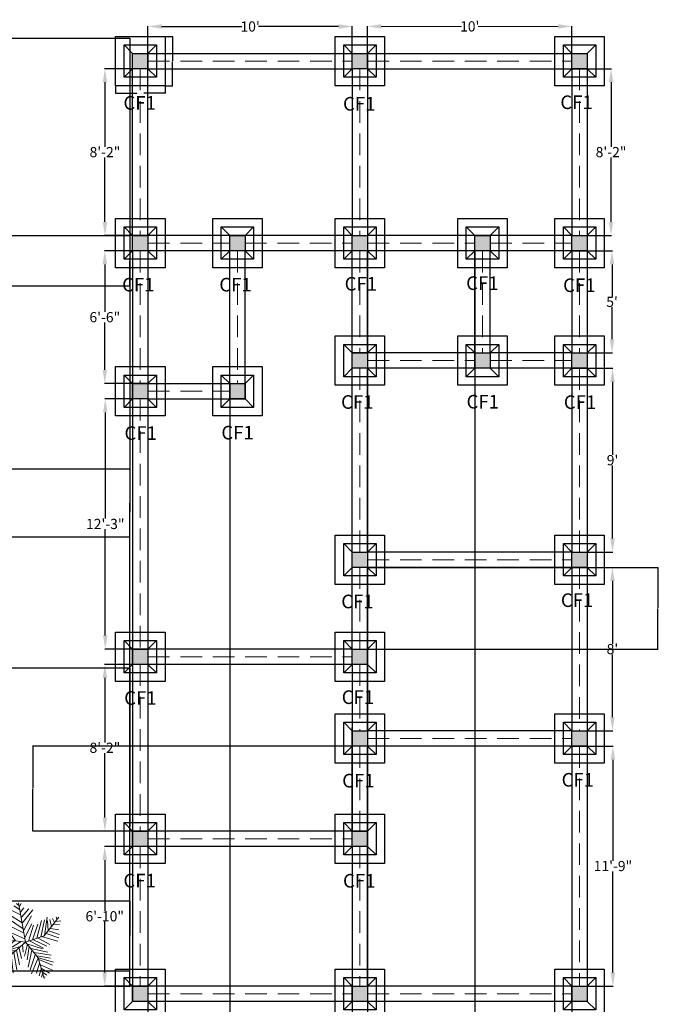
# Model space of a CAD drawing. Units: inches. Extents: x 37 to 824, y -700 to 234.
# Tile 77 of 77: x 449 to 824, y -377 to 202. Entities that reach past the tile are written whole.
import ezdxf

# ---------------------------------------------------------------- set-up
doc = ezdxf.new("R2010")
doc.units = ezdxf.units.IN
doc.header["$MEASUREMENT"] = 0
doc.linetypes.add('DASHED', pattern=[19.05, 12.7, -6.35])
for name, color, linetype, lineweight in [('A-ANNO-DIMS', 2, 'Continuous', 18), ('A-ANNO-TEXT', 7, 'Continuous', 18), ('A-SITE-PLNT', 3, 'Continuous', 13), ('S-BEAM', 4, 'Continuous', 25), ('S-BEAM-CNTR', 220, 'DASHED', 18), ('S-COLS', 2, 'Continuous', 35), ('S-FNDN', 220, 'Continuous', 25)]:
    doc.layers.add(name, color=color, linetype=linetype, lineweight=lineweight)
doc.styles.get("Standard").update_dxf_attribs({"font": 'arial.ttf'})
doc.dimstyles.get("Standard").update_dxf_attribs({"dimtxt": 0.18, "dimasz": 0.18, "dimexe": 0.18, "dimexo": 0.0625, "dimgap": 0.09, "dimtad": 0, "dimtih": 1, "dimtoh": 1, "dimdec": 1, "dimzin": 0, "dimdsep": 46, "dimlunit": 4, "dimtxsty": 'Standard', "dimcen": 0.09, "dimadec": 0, "dimazin": 0, "dimtfac": 1, "dimtdec": 1, "dimtofl": 0, "dimtmove": 0, "dimatfit": 3, "dimfxl": 1, "dimtolj": 1, "dimtzin": 0, "dimarcsym": 0})

# ---------------------------------------------------------------- blocks, each defined once
blk = doc.blocks.new('*D12')
at = {"layer": 'A-ANNO-DIMS', "color": 0, "lineweight": -2, "ltscale": 0.5, "transparency": 16777216}
for p, q in [((524.2, 173.16), (524.2, 198.08)), ((532.2, 197.9), (579.3, 197.9)), ((636.2, 197.9), (589.1, 197.9)), ((644.2, 173.16), (644.2, 198.08))]:
    blk.add_line(p, q, dxfattribs=at)
at = {"layer": 'A-ANNO-DIMS', "color": 0, "ltscale": 0.5, "transparency": 16777216}
for points in [[(532.2, 199.23), (532.2, 196.56), (524.2, 197.9)], [(636.2, 199.23), (636.2, 196.56), (644.2, 197.9)]]:
    blk.add_solid(points, dxfattribs=at)
at = {"layer": 'Defpoints', "color": 0, "ltscale": 0.5, "transparency": 16777216}
for p in [(644.2, 197.9), (524.2, 173.09), (644.2, 173.09)]:
    blk.add_point(p, dxfattribs=at)
at = {"layer": 'A-ANNO-DIMS', "color": 0, "ltscale": 0.5, "transparency": 16777216, "insert": (584.2, 197.9), "char_height": 6, "attachment_point": 5}
blk.add_mtext("\\A1;10'", dxfattribs=at)
blk = doc.blocks.new('*D13')
at = {"layer": 'A-ANNO-DIMS', "color": 0, "lineweight": -2, "ltscale": 0.5, "transparency": 16777216}
for p, q in [((653.2, 173.16), (653.2, 198.13)), ((773.2, 173.16), (773.2, 198.13))]:
    blk.add_line(p, q, dxfattribs=at)
at = {"layer": 'A-ANNO-DIMS', "color": 0, "ltscale": 0.5, "transparency": 16777216}
for p, q in [((661.2, 197.95), (708.3, 197.95)), ((765.2, 197.95), (718.1, 197.95))]:
    blk.add_line(p, q, dxfattribs=at)
for points in [[(661.2, 199.28), (661.2, 196.62), (653.2, 197.95)], [(765.2, 199.28), (765.2, 196.62), (773.2, 197.95)]]:
    blk.add_solid(points, dxfattribs=at)
at = {"layer": 'Defpoints', "color": 0, "ltscale": 0.5, "transparency": 16777216}
for p in [(773.2, 197.95), (653.2, 173.09), (773.2, 173.09)]:
    blk.add_point(p, dxfattribs=at)
at = {"layer": 'A-ANNO-DIMS', "color": 0, "ltscale": 0.5, "transparency": 16777216, "insert": (713.2, 197.95), "char_height": 6, "attachment_point": 5}
blk.add_mtext("\\A1;10'", dxfattribs=at)
blk = doc.blocks.new('*D14')
at = {"layer": 'A-ANNO-DIMS', "color": 0, "lineweight": -2, "ltscale": 0.5, "transparency": 16777216}
for p, q in [((773.26, 173.09), (796.39, 173.09)), ((796.21, 165.09), (796.21, 127.25)), ((796.21, 83.09), (796.21, 120.94)), ((773.26, 75.09), (796.39, 75.09))]:
    blk.add_line(p, q, dxfattribs=at)
at = {"layer": 'A-ANNO-DIMS', "color": 0, "ltscale": 0.5, "transparency": 16777216}
for points in [[(794.88, 165.09), (797.55, 165.09), (796.21, 173.09)], [(794.88, 83.09), (797.55, 83.09), (796.21, 75.09)]]:
    blk.add_solid(points, dxfattribs=at)
at = {"layer": 'Defpoints', "color": 0, "ltscale": 0.5, "transparency": 16777216}
for p in [(773.2, 173.09), (773.2, 75.09), (796.21, 75.09)]:
    blk.add_point(p, dxfattribs=at)
at = {"layer": 'A-ANNO-DIMS', "color": 0, "ltscale": 0.5, "transparency": 16777216, "insert": (796.21, 124.09), "char_height": 6, "attachment_point": 5}
blk.add_mtext('\\A1;8\'-2"', dxfattribs=at)
blk = doc.blocks.new('*D15')
at = {"layer": 'A-ANNO-DIMS', "color": 0, "lineweight": -2, "ltscale": 0.6, "transparency": 16777216}
for p, q in [((773.26, 66.09), (796.98, 66.09)), ((796.8, 58.09), (796.8, 39.23)), ((796.8, 14.09), (796.8, 32.95)), ((773.26, 6.09), (796.98, 6.09))]:
    blk.add_line(p, q, dxfattribs=at)
at = {"layer": 'A-ANNO-DIMS', "color": 0, "ltscale": 0.6, "transparency": 16777216}
for points in [[(795.47, 58.09), (798.13, 58.09), (796.8, 66.09)], [(795.47, 14.09), (798.13, 14.09), (796.8, 6.09)]]:
    blk.add_solid(points, dxfattribs=at)
at = {"layer": 'Defpoints', "color": 0, "ltscale": 0.6, "transparency": 16777216}
for p in [(773.2, 66.09), (773.2, 6.09), (796.8, 6.09)]:
    blk.add_point(p, dxfattribs=at)
at = {"layer": 'A-ANNO-DIMS', "color": 0, "ltscale": 0.6, "transparency": 16777216, "insert": (796.8, 36.09), "char_height": 6, "attachment_point": 5}
blk.add_mtext("\\A1;5'", dxfattribs=at)
blk = doc.blocks.new('*D16')
at = {"layer": 'A-ANNO-DIMS', "color": 0, "lineweight": -2, "ltscale": 0.5, "transparency": 16777216}
for p, q in [((773.26, -2.91), (797.27, -2.91)), ((797.09, -10.91), (797.09, -53.75)), ((797.09, -102.91), (797.09, -60.06)), ((773.26, -110.91), (797.27, -110.91))]:
    blk.add_line(p, q, dxfattribs=at)
at = {"layer": 'A-ANNO-DIMS', "color": 0, "ltscale": 0.5, "transparency": 16777216}
for points in [[(795.75, -10.91), (798.42, -10.91), (797.09, -2.91)], [(795.75, -102.91), (798.42, -102.91), (797.09, -110.91)]]:
    blk.add_solid(points, dxfattribs=at)
at = {"layer": 'Defpoints', "color": 0, "ltscale": 0.5, "transparency": 16777216}
for p in [(773.2, -2.91), (773.2, -110.91), (797.09, -110.91)]:
    blk.add_point(p, dxfattribs=at)
at = {"layer": 'A-ANNO-DIMS', "color": 0, "ltscale": 0.5, "transparency": 16777216, "insert": (797.09, -56.91), "char_height": 6, "attachment_point": 5}
blk.add_mtext("\\A1;9'", dxfattribs=at)
blk = doc.blocks.new('*D17')
at = {"layer": 'A-ANNO-DIMS', "color": 0, "lineweight": -2, "ltscale": 0.5, "transparency": 16777216}
for p, q in [((773.26, -119.91), (797.22, -119.91)), ((797.04, -127.91), (797.04, -164.75)), ((797.04, -207.91), (797.04, -171.06)), ((773.26, -215.91), (797.22, -215.91))]:
    blk.add_line(p, q, dxfattribs=at)
at = {"layer": 'A-ANNO-DIMS', "color": 0, "ltscale": 0.5, "transparency": 16777216}
for points in [[(795.71, -127.91), (798.37, -127.91), (797.04, -119.91)], [(795.71, -207.91), (798.37, -207.91), (797.04, -215.91)]]:
    blk.add_solid(points, dxfattribs=at)
at = {"layer": 'Defpoints', "color": 0, "ltscale": 0.5, "transparency": 16777216}
for p in [(773.2, -119.91), (773.2, -215.91), (797.04, -215.91)]:
    blk.add_point(p, dxfattribs=at)
at = {"layer": 'A-ANNO-DIMS', "color": 0, "ltscale": 0.5, "transparency": 16777216, "insert": (797.04, -167.91), "char_height": 6, "attachment_point": 5}
blk.add_mtext("\\A1;8'", dxfattribs=at)
blk = doc.blocks.new('*D18')
at = {"layer": 'A-ANNO-DIMS', "color": 0, "lineweight": -2, "ltscale": 0.5, "transparency": 16777216}
for p, q in [((773.26, -224.91), (797.49, -224.91)), ((797.31, -232.91), (797.31, -292.25)), ((797.31, -357.91), (797.31, -298.56)), ((773.26, -365.91), (797.49, -365.91))]:
    blk.add_line(p, q, dxfattribs=at)
at = {"layer": 'A-ANNO-DIMS', "color": 0, "ltscale": 0.5, "transparency": 16777216}
for points in [[(795.98, -232.91), (798.65, -232.91), (797.31, -224.91)], [(795.98, -357.91), (798.65, -357.91), (797.31, -365.91)]]:
    blk.add_solid(points, dxfattribs=at)
at = {"layer": 'Defpoints', "color": 0, "ltscale": 0.5, "transparency": 16777216}
for p in [(773.2, -224.91), (773.2, -365.91), (797.31, -365.91)]:
    blk.add_point(p, dxfattribs=at)
at = {"layer": 'A-ANNO-DIMS', "color": 0, "ltscale": 0.5, "transparency": 16777216, "insert": (797.31, -295.41), "char_height": 6, "attachment_point": 5}
blk.add_mtext('\\A1;11\'-9"', dxfattribs=at)
blk = doc.blocks.new('*D19')
at = {"layer": 'A-ANNO-DIMS', "color": 0, "lineweight": -2, "ltscale": 0.5, "transparency": 16777216}
for p, q in [((524.14, 173.09), (498.75, 173.09)), ((498.93, 165.09), (498.93, 127.25)), ((498.93, 83.09), (498.93, 120.94)), ((524.14, 75.09), (498.75, 75.09))]:
    blk.add_line(p, q, dxfattribs=at)
at = {"layer": 'A-ANNO-DIMS', "color": 0, "ltscale": 0.5, "transparency": 16777216}
for points in [[(497.6, 165.09), (500.27, 165.09), (498.93, 173.09)], [(497.6, 83.09), (500.27, 83.09), (498.93, 75.09)]]:
    blk.add_solid(points, dxfattribs=at)
at = {"layer": 'Defpoints', "color": 0, "ltscale": 0.5, "transparency": 16777216}
for p in [(524.2, 173.09), (498.93, 75.09), (524.2, 75.09)]:
    blk.add_point(p, dxfattribs=at)
at = {"layer": 'A-ANNO-DIMS', "color": 0, "ltscale": 0.5, "transparency": 16777216, "insert": (498.93, 124.09), "char_height": 6, "attachment_point": 5}
blk.add_mtext('\\A1;8\'-2"', dxfattribs=at)
blk = doc.blocks.new('*D20')
at = {"layer": 'A-ANNO-DIMS', "color": 0, "lineweight": -2, "ltscale": 0.5, "transparency": 16777216}
for p, q in [((524.14, 66.09), (498.66, 66.09)), ((498.84, 58.09), (498.84, 30.25)), ((498.84, -3.91), (498.84, 23.94)), ((524.14, -11.91), (498.66, -11.91))]:
    blk.add_line(p, q, dxfattribs=at)
at = {"layer": 'A-ANNO-DIMS', "color": 0, "ltscale": 0.5, "transparency": 16777216}
for points in [[(497.5, 58.09), (500.17, 58.09), (498.84, 66.09)], [(497.5, -3.91), (500.17, -3.91), (498.84, -11.91)]]:
    blk.add_solid(points, dxfattribs=at)
at = {"layer": 'Defpoints', "color": 0, "ltscale": 0.5, "transparency": 16777216}
for p in [(524.2, 66.09), (498.84, -11.91), (524.2, -11.91)]:
    blk.add_point(p, dxfattribs=at)
at = {"layer": 'A-ANNO-DIMS', "color": 0, "ltscale": 0.5, "transparency": 16777216, "insert": (498.84, 27.09), "char_height": 6, "attachment_point": 5}
blk.add_mtext('\\A1;6\'-6"', dxfattribs=at)
blk = doc.blocks.new('*D21')
at = {"layer": 'A-ANNO-DIMS', "color": 0, "lineweight": -2, "ltscale": 0.5, "transparency": 16777216}
for p, q in [((524.14, -20.91), (498.92, -20.91)), ((499.1, -28.91), (499.1, -91.25)), ((499.1, -159.91), (499.1, -97.56)), ((524.14, -167.91), (498.92, -167.91))]:
    blk.add_line(p, q, dxfattribs=at)
at = {"layer": 'A-ANNO-DIMS', "color": 0, "ltscale": 0.5, "transparency": 16777216}
for points in [[(497.77, -28.91), (500.44, -28.91), (499.1, -20.91)], [(497.77, -159.91), (500.44, -159.91), (499.1, -167.91)]]:
    blk.add_solid(points, dxfattribs=at)
at = {"layer": 'Defpoints', "color": 0, "ltscale": 0.5, "transparency": 16777216}
for p in [(524.2, -20.91), (499.1, -167.91), (524.2, -167.91)]:
    blk.add_point(p, dxfattribs=at)
at = {"layer": 'A-ANNO-DIMS', "color": 0, "ltscale": 0.5, "transparency": 16777216, "insert": (499.1, -94.41), "char_height": 6, "attachment_point": 5}
blk.add_mtext('\\A1;12\'-3"', dxfattribs=at)
blk = doc.blocks.new('*D22')
at = {"layer": 'A-ANNO-DIMS', "color": 0, "lineweight": -2, "ltscale": 0.5, "transparency": 16777216}
for p, q in [((524.14, -176.91), (498.72, -176.91)), ((498.9, -184.91), (498.9, -222.75)), ((498.9, -266.91), (498.9, -229.06)), ((524.14, -274.91), (498.72, -274.91))]:
    blk.add_line(p, q, dxfattribs=at)
at = {"layer": 'A-ANNO-DIMS', "color": 0, "ltscale": 0.5, "transparency": 16777216}
for points in [[(497.56, -184.91), (500.23, -184.91), (498.9, -176.91)], [(497.56, -266.91), (500.23, -266.91), (498.9, -274.91)]]:
    blk.add_solid(points, dxfattribs=at)
at = {"layer": 'Defpoints', "color": 0, "ltscale": 0.5, "transparency": 16777216}
for p in [(524.2, -176.91), (498.9, -274.91), (524.2, -274.91)]:
    blk.add_point(p, dxfattribs=at)
at = {"layer": 'A-ANNO-DIMS', "color": 0, "ltscale": 0.5, "transparency": 16777216, "insert": (498.9, -225.91), "char_height": 6, "attachment_point": 5}
blk.add_mtext('\\A1;8\'-2"', dxfattribs=at)
blk = doc.blocks.new('*D23')
at = {"layer": 'A-ANNO-DIMS', "color": 0, "lineweight": -2, "ltscale": 0.5, "transparency": 16777216}
for p, q in [((524.14, -283.91), (498.61, -283.91)), ((498.79, -291.91), (498.79, -321.75)), ((498.79, -357.91), (498.79, -328.06)), ((524.14, -365.91), (498.61, -365.91))]:
    blk.add_line(p, q, dxfattribs=at)
at = {"layer": 'A-ANNO-DIMS', "color": 0, "ltscale": 0.5, "transparency": 16777216}
for points in [[(497.46, -291.91), (500.12, -291.91), (498.79, -283.91)], [(497.46, -357.91), (500.12, -357.91), (498.79, -365.91)]]:
    blk.add_solid(points, dxfattribs=at)
at = {"layer": 'Defpoints', "color": 0, "ltscale": 0.5, "transparency": 16777216}
for p in [(524.2, -283.91), (498.79, -365.91), (524.2, -365.91)]:
    blk.add_point(p, dxfattribs=at)
at = {"layer": 'A-ANNO-DIMS', "color": 0, "ltscale": 0.5, "transparency": 16777216, "insert": (498.79, -324.91), "char_height": 6, "attachment_point": 5}
blk.add_mtext('\\A1;6\'-10"', dxfattribs=at)
blk = doc.blocks.new('*D24')
at = {"layer": 'A-ANNO-DIMS', "color": 0, "lineweight": -2, "ltscale": 0.5, "transparency": 16777216}
for p, q in [((524.2, -365.97), (524.2, -389.77)), ((644.2, -365.97), (644.2, -389.77)), ((532.2, -389.59), (579.3, -389.59)), ((636.2, -389.59), (589.1, -389.59))]:
    blk.add_line(p, q, dxfattribs=at)
at = {"layer": 'A-ANNO-DIMS', "color": 0, "ltscale": 0.5, "transparency": 16777216}
for points in [[(532.2, -388.25), (532.2, -390.92), (524.2, -389.59)], [(636.2, -388.25), (636.2, -390.92), (644.2, -389.59)]]:
    blk.add_solid(points, dxfattribs=at)
at = {"layer": 'Defpoints', "color": 0, "ltscale": 0.5, "transparency": 16777216}
for p in [(524.2, -365.91), (644.2, -365.91), (644.2, -389.59)]:
    blk.add_point(p, dxfattribs=at)
at = {"layer": 'A-ANNO-DIMS', "color": 0, "ltscale": 0.5, "transparency": 16777216, "insert": (584.2, -389.59), "char_height": 6, "attachment_point": 5}
blk.add_mtext("\\A1;10'", dxfattribs=at)
blk = doc.blocks.new('*D25')
at = {"layer": 'A-ANNO-DIMS', "color": 0, "lineweight": -2, "ltscale": 0.5, "transparency": 16777216}
for p, q in [((653.2, -365.97), (653.2, -390.17)), ((773.2, -365.97), (773.2, -390.17)), ((661.2, -389.99), (708.3, -389.99)), ((765.2, -389.99), (718.1, -389.99))]:
    blk.add_line(p, q, dxfattribs=at)
at = {"layer": 'A-ANNO-DIMS', "color": 0, "ltscale": 0.5, "transparency": 16777216}
for points in [[(661.2, -388.65), (661.2, -391.32), (653.2, -389.99)], [(765.2, -388.65), (765.2, -391.32), (773.2, -389.99)]]:
    blk.add_solid(points, dxfattribs=at)
at = {"layer": 'Defpoints', "color": 0, "ltscale": 0.5, "transparency": 16777216}
for p in [(653.2, -365.91), (773.2, -365.91), (773.2, -389.99)]:
    blk.add_point(p, dxfattribs=at)
at = {"layer": 'A-ANNO-DIMS', "color": 0, "ltscale": 0.5, "transparency": 16777216, "insert": (713.2, -389.99), "char_height": 6, "attachment_point": 5}
blk.add_mtext("\\A1;10'", dxfattribs=at)
blk = doc.blocks.new('*U33')
for p, q in [((0, 0), (-10.5, 57)), ((-7.288, 39.707), (-21.778, 46.673)), ((-8.737, 47.138), (-17.069, 52.711)), ((-10.186, 53.64), (-13.084, 55.962)), ((-9.099, 51.782), (-6.563, 55.962)), ((-7.65, 43.423), (-2.578, 49.46)), ((-5.839, 35.992), (4.667, 48.067)), ((-5.114, 27.632), (10.463, 46.673)), ((-48.585, 21.131), (-49.309, 29.026)), ((-43.513, 28.561), (-42.427, 15.558)), ((-3.665, 19.273), (-27.574, 35.527)), ((-5.114, 28.097), (-24.676, 40.636)), ((-2.941, 16.486), (8.652, 37.85)), ((16.259, 5.805), (23.142, 31.348)), ((22.055, 7.198), (27.489, 32.277)), ((27, 9), (48, 36)), ((27.127, 9.056), (31.112, 35.992)), ((31.836, 30.883), (32.561, 16.486)), ((35.096, 32.741), (37.27, 22.524)), ((38.719, 34.134), (41.979, 28.561)), ((43.791, 29.954), (51.036, 30.883)), ((44.153, 36.456), (45.239, 32.741)), ((-47.498, 19.737), (-55.83, 18.344)), ((-31.5, 4.5), (-52.5, 25.5)), ((-38.442, 26.239), (-34.819, 7.663)), ((-35.544, 28.097), (-24.314, 3.947)), ((-14.533, 2.09), (-30.834, 25.31)), ((-24.314, 23.917), (-2.941, 13.7)), ((-1.129, 6.734), (9.014, 26.704)), ((3.942, 1.625), (11.187, 24.381)), ((10.101, 3.483), (17.708, 26.239)), ((33.285, 16.486), (48.862, 10.913)), ((36.183, 19.737), (48.137, 17.88)), ((40.53, 25.775), (48.862, 24.846)), ((-40.615, 13.7), (-55.105, 10.913)), ((-33.37, 6.269), (-52.207, 5.34)), ((-28.299, 3.483), (-47.86, -5.805)), ((-21.416, 3.018), (-38.079, -8.128)), ((0, 0), (-31.5, 4.5)), ((-15.982, 2.09), (-30.11, -9.521)), ((0, 0), (-22.5, -19.5)), ((-6.563, 1.161), (-21.416, -8.128)), ((-20.691, 13.7), (-1.129, 4.876)), ((0, 0), (27, 9)), ((0, 0), (18, -22.5)), ((6.478, 1.625), (26.04, -8.592)), ((11.187, 3.483), (30.749, -5.805)), ((18.07, 5.805), (35.096, -3.483)), ((24.229, 7.663), (46.688, 1.625)), ((29.662, 12.307), (48.137, 6.269)), ((-15.257, -12.772), (-30.11, -12.772)), ((-6.563, -5.805), (-19.967, -9.985)), ((-13.446, -11.378), (-8.737, -32.741)), ((-9.461, -8.592), (-6.201, -23.453)), ((-4.752, -3.483), (-3.665, -14.629)), ((2.493, -3.019), (-1.491, -20.202)), ((1.769, -2.555), (24.229, -9.521)), ((5.029, -6.27), (2.131, -25.775)), ((9.014, -11.378), (3.58, -35.992)), ((7.565, -9.056), (32.198, -14.629)), ((-17.431, -15.094), (-42.789, -18.809)), ((-24.314, -21.596), (-42.427, -22.06)), ((-26.849, -26.24), (-40.253, -25.775)), ((-22.5, -19.5), (-37.5, -45)), ((-25.038, -23.918), (-22.865, -45.281)), ((-20.691, -18.345), (-17.793, -44.352)), ((-17.069, -15.094), (-12.721, -40.172)), ((14.085, -16.951), (6.478, -40.172)), ((18.07, -22.524), (8.289, -45.745)), ((12.274, -15.094), (36.907, -18.809)), ((16.259, -19.738), (36.183, -22.989)), ((18, -22.5), (27, -52.5)), ((18.433, -22.524), (40.53, -29.026)), ((19.157, -25.311), (38.719, -33.206)), ((-28.299, -29.026), (-42.789, -31.348)), ((-30.834, -34.135), (-42.427, -35.528)), ((-34.457, -39.708), (-40.978, -42.494)), ((-32.646, -36.921), (-31.921, -44.352)), ((-29.023, -30.884), (-27.936, -43.887)), ((20.244, -30.419), (15.897, -44.816)), ((22.78, -37.85), (19.519, -48.532)), ((21.331, -32.741), (39.081, -40.636)), ((22.78, -38.314), (34.372, -44.816)), ((24.591, -45.745), (23.142, -50.854)), ((24.591, -43.423), (30.749, -47.603)), ((26.764, -49.925), (28.213, -50.854))]:
    blk.add_line(p, q)
blk = doc.blocks.new('FOOTING-CF1')
at = {"ltscale": 0.6}
for p, q in [((0, 29), (29, 29)), ((0, 0), (0, 29)), ((29, 29), (29, 0)), ((29, 0), (0, 0))]:
    blk.add_line(p, q, dxfattribs=at)
for p, q in [((5, 24), (24, 24)), ((5, 5), (5, 24)), ((5, 24), (10, 19)), ((19, 19), (24, 24)), ((24, 24), (24, 5)), ((10, 19), (19, 19)), ((10, 10), (10, 19)), ((19, 19), (19, 10)), ((5, 5), (10, 10)), ((19, 10), (10, 10)), ((24, 5), (19, 10)), ((24, 5), (5, 5))]:
    blk.add_line(p, q)
blk = doc.blocks.new('*D42')
at = {"layer": 'A-ANNO-DIMS', "color": 0, "lineweight": -2, "ltscale": 0.5, "transparency": 16777216}
for p, q in [((505.2, 163.03), (505.2, 158.56)), ((534.2, 163.03), (534.2, 158.56)), ((505.38, 158.74), (517.6, 158.74)), ((534.02, 158.74), (521.8, 158.74))]:
    blk.add_line(p, q, dxfattribs=at)
at = {"layer": 'A-ANNO-DIMS', "color": 0, "ltscale": 0.5, "transparency": 16777216}
for points in [[(505.38, 158.77), (505.38, 158.71), (505.2, 158.74)], [(534.02, 158.77), (534.02, 158.71), (534.2, 158.74)]]:
    blk.add_solid(points, dxfattribs=at)
at = {"layer": 'Defpoints', "color": 0, "ltscale": 0.5, "transparency": 16777216}
for p in [(505.2, 163.09), (534.2, 163.09), (534.2, 158.74)]:
    blk.add_point(p, dxfattribs=at)
at = {"layer": 'A-ANNO-DIMS', "color": 0, "ltscale": 0.5, "transparency": 16777216, "insert": (519.7, 158.74), "char_height": 0.18, "attachment_point": 5}
blk.add_mtext('\\A1;COLUMN FOOTING CF1 2\'-5" TYP.', dxfattribs=at)
blk = doc.blocks.new('*D43')
at = {"layer": 'A-ANNO-DIMS', "color": 0, "lineweight": -2, "ltscale": 0.5, "transparency": 16777216}
for p, q in [((534.26, 192.09), (538.73, 192.09)), ((538.55, 191.91), (538.55, 177.77)), ((538.55, 163.27), (538.55, 177.41)), ((534.26, 163.09), (538.73, 163.09))]:
    blk.add_line(p, q, dxfattribs=at)
at = {"layer": 'A-ANNO-DIMS', "color": 0, "ltscale": 0.5, "transparency": 16777216}
for points in [[(538.52, 191.91), (538.58, 191.91), (538.55, 192.09)], [(538.52, 163.27), (538.58, 163.27), (538.55, 163.09)]]:
    blk.add_solid(points, dxfattribs=at)
at = {"layer": 'Defpoints', "color": 0, "ltscale": 0.5, "transparency": 16777216}
for p in [(534.2, 192.09), (538.55, 192.09), (534.2, 163.09)]:
    blk.add_point(p, dxfattribs=at)
at = {"layer": 'A-ANNO-DIMS', "color": 0, "ltscale": 0.5, "transparency": 16777216, "insert": (538.55, 177.59), "char_height": 0.18, "attachment_point": 5}
blk.add_mtext('\\A1;2\'-5" TYP.', dxfattribs=at)
blk = doc.blocks.new('*D64')
at = {"layer": 'A-ANNO-DIMS', "color": 0, "lineweight": -2, "ltscale": 0.5, "transparency": 16777216}
for p, q in [((428.14, 191.09), (513.77, 191.09)), ((513.59, 190.91), (513.59, -87.23)), ((513.59, -365.73), (513.59, -87.59)), ((428.14, -365.91), (513.77, -365.91))]:
    blk.add_line(p, q, dxfattribs=at)
at = {"layer": 'A-ANNO-DIMS', "color": 0, "ltscale": 0.5, "transparency": 16777216}
for points in [[(513.56, 190.91), (513.62, 190.91), (513.59, 191.09)], [(513.56, -365.73), (513.62, -365.73), (513.59, -365.91)]]:
    blk.add_solid(points, dxfattribs=at)
at = {"layer": 'Defpoints', "color": 0, "ltscale": 0.5, "transparency": 16777216}
for p in [(428.08, 191.09), (428.08, -365.91), (513.59, -365.91)]:
    blk.add_point(p, dxfattribs=at)
at = {"layer": 'A-ANNO-DIMS', "color": 0, "ltscale": 0.5, "transparency": 16777216, "insert": (513.59, -87.41), "char_height": 0.18, "attachment_point": 5}
blk.add_mtext('\\A1;46\'-5"', dxfattribs=at)
blk = doc.blocks.new('*D65')
at = {"layer": 'A-ANNO-DIMS', "color": 0, "lineweight": -2, "ltscale": 0.5, "transparency": 16777216}
for p, q in [((428.14, -178.91), (513.77, -178.91)), ((513.59, -179.09), (513.59, -272.23)), ((513.59, -365.73), (513.59, -272.59)), ((428.14, -365.91), (513.77, -365.91))]:
    blk.add_line(p, q, dxfattribs=at)
at = {"layer": 'A-ANNO-DIMS', "color": 0, "ltscale": 0.5, "transparency": 16777216}
for points in [[(513.56, -179.09), (513.62, -179.09), (513.59, -178.91)], [(513.56, -365.73), (513.62, -365.73), (513.59, -365.91)]]:
    blk.add_solid(points, dxfattribs=at)
at = {"layer": 'Defpoints', "color": 0, "ltscale": 0.5, "transparency": 16777216}
for p in [(428.08, -178.91), (428.08, -365.91), (513.59, -365.91)]:
    blk.add_point(p, dxfattribs=at)
at = {"layer": 'A-ANNO-DIMS', "color": 0, "ltscale": 0.5, "transparency": 16777216, "insert": (513.59, -272.41), "char_height": 0.18, "attachment_point": 5}
blk.add_mtext('\\A1;15\'-7"', dxfattribs=at)
blk = doc.blocks.new('*D76')
at = {"layer": 'A-ANNO-DIMS', "color": 0, "lineweight": -2, "ltscale": 0.5, "transparency": 16777216}
for p, q in [((227.14, 75.09), (513.77, 75.09)), ((513.59, 74.91), (513.59, 60.51)), ((513.59, 45.74), (513.59, 60.14)), ((227.14, 45.56), (513.77, 45.56))]:
    blk.add_line(p, q, dxfattribs=at)
at = {"layer": 'A-ANNO-DIMS', "color": 0, "ltscale": 0.5, "transparency": 16777216}
for points in [[(513.56, 74.91), (513.62, 74.91), (513.59, 75.09)], [(513.56, 45.74), (513.62, 45.74), (513.59, 45.56)]]:
    blk.add_solid(points, dxfattribs=at)
at = {"layer": 'Defpoints', "color": 0, "ltscale": 0.5, "transparency": 16777216}
for p in [(227.08, 75.09), (227.08, 45.56), (513.59, 45.56)]:
    blk.add_point(p, dxfattribs=at)
at = {"layer": 'A-ANNO-DIMS', "color": 0, "ltscale": 0.5, "transparency": 16777216, "insert": (513.59, 60.33), "char_height": 0.18, "attachment_point": 5}
blk.add_mtext('\\A1;2\'-5 1/2"', dxfattribs=at)
blk = doc.blocks.new('*D79')
at = {"layer": 'A-ANNO-DIMS', "color": 0, "lineweight": -2, "ltscale": 0.5, "transparency": 16777216}
for p, q in [((299.14, -62.02), (513.77, -62.02)), ((513.59, -62.2), (513.59, -81.78)), ((513.59, -101.73), (513.59, -82.15)), ((296.14, -101.91), (513.77, -101.91))]:
    blk.add_line(p, q, dxfattribs=at)
at = {"layer": 'A-ANNO-DIMS', "color": 0, "ltscale": 0.5, "transparency": 16777216}
for points in [[(513.56, -62.2), (513.62, -62.2), (513.59, -62.02)], [(513.56, -101.73), (513.62, -101.73), (513.59, -101.91)]]:
    blk.add_solid(points, dxfattribs=at)
at = {"layer": 'Defpoints', "color": 0, "ltscale": 0.5, "transparency": 16777216}
for p in [(299.08, -62.02), (296.08, -101.91), (513.59, -101.91)]:
    blk.add_point(p, dxfattribs=at)
at = {"layer": 'A-ANNO-DIMS', "color": 0, "ltscale": 0.5, "transparency": 16777216, "insert": (513.59, -81.97), "char_height": 0.18, "attachment_point": 5}
blk.add_mtext('\\A1;3\'-4"', dxfattribs=at)
blk = doc.blocks.new('*D88')
at = {"layer": 'A-ANNO-DIMS', "color": 0, "lineweight": -2, "ltscale": 0.5, "transparency": 16777216}
for p, q in [((296.14, -315.91), (513.77, -315.91)), ((513.59, -316.09), (513.59, -336.23)), ((513.59, -356.73), (513.59, -336.59)), ((296.14, -356.91), (513.77, -356.91))]:
    blk.add_line(p, q, dxfattribs=at)
at = {"layer": 'A-ANNO-DIMS', "color": 0, "ltscale": 0.5, "transparency": 16777216}
for points in [[(513.56, -316.09), (513.62, -316.09), (513.59, -315.91)], [(513.56, -356.73), (513.62, -356.73), (513.59, -356.91)]]:
    blk.add_solid(points, dxfattribs=at)
at = {"layer": 'Defpoints', "color": 0, "ltscale": 0.5, "transparency": 16777216}
for p in [(296.08, -315.91), (296.08, -356.91), (513.59, -356.91)]:
    blk.add_point(p, dxfattribs=at)
at = {"layer": 'A-ANNO-DIMS', "color": 0, "ltscale": 0.5, "transparency": 16777216, "insert": (513.59, -336.41), "char_height": 0.18, "attachment_point": 5}
blk.add_mtext('\\A1;3\'-5"', dxfattribs=at)
blk = doc.blocks.new('*D90')
at = {"layer": 'A-ANNO-DIMS', "color": 0, "lineweight": -2, "ltscale": 0.5, "transparency": 16777216}
for p, q in [((524.2, -11.97), (524.2, -450)), ((572.2, -11.97), (572.2, -450)), ((524.38, -449.82), (547.87, -449.82)), ((572.02, -449.82), (548.53, -449.82))]:
    blk.add_line(p, q, dxfattribs=at)
at = {"layer": 'A-ANNO-DIMS', "color": 0, "ltscale": 0.5, "transparency": 16777216}
for points in [[(524.38, -449.79), (524.38, -449.85), (524.2, -449.82)], [(572.02, -449.79), (572.02, -449.85), (572.2, -449.82)]]:
    blk.add_solid(points, dxfattribs=at)
at = {"layer": 'Defpoints', "color": 0, "ltscale": 0.5, "transparency": 16777216}
for p in [(524.2, -11.91), (572.2, -11.91), (572.2, -449.82)]:
    blk.add_point(p, dxfattribs=at)
at = {"layer": 'A-ANNO-DIMS', "color": 0, "ltscale": 0.5, "transparency": 16777216, "insert": (548.2, -449.82), "char_height": 0.18, "attachment_point": 5}
blk.add_mtext('\\A1;4\'-0"', dxfattribs=at)
blk = doc.blocks.new('*D91')
at = {"layer": 'A-ANNO-DIMS', "color": 0, "lineweight": -2, "ltscale": 0.5, "transparency": 16777216}
for p, q in [((653.2, 66.03), (653.2, -450)), ((716.2, 66.03), (716.2, -450)), ((653.38, -449.82), (684.37, -449.82)), ((716.02, -449.82), (685.03, -449.82))]:
    blk.add_line(p, q, dxfattribs=at)
at = {"layer": 'A-ANNO-DIMS', "color": 0, "ltscale": 0.5, "transparency": 16777216}
for points in [[(653.38, -449.79), (653.38, -449.85), (653.2, -449.82)], [(716.02, -449.79), (716.02, -449.85), (716.2, -449.82)]]:
    blk.add_solid(points, dxfattribs=at)
at = {"layer": 'Defpoints', "color": 0, "ltscale": 0.5, "transparency": 16777216}
for p in [(653.2, 66.09), (716.2, 66.09), (716.2, -449.82)]:
    blk.add_point(p, dxfattribs=at)
at = {"layer": 'A-ANNO-DIMS', "color": 0, "ltscale": 0.5, "transparency": 16777216, "insert": (684.7, -449.82), "char_height": 0.18, "attachment_point": 5}
blk.add_mtext('\\A1;5\'-3"', dxfattribs=at)
blk = doc.blocks.new('*D92')
at = {"layer": 'A-ANNO-DIMS', "color": 0, "lineweight": -2, "ltscale": 0.5, "transparency": 16777216}
for p, q in [((653.26, -119.91), (823.88, -119.91)), ((823.7, -120.09), (823.7, -143.73)), ((823.7, -167.73), (823.7, -144.09)), ((653.26, -167.91), (823.88, -167.91))]:
    blk.add_line(p, q, dxfattribs=at)
at = {"layer": 'A-ANNO-DIMS', "color": 0, "ltscale": 0.5, "transparency": 16777216}
for points in [[(823.67, -120.09), (823.73, -120.09), (823.7, -119.91)], [(823.67, -167.73), (823.73, -167.73), (823.7, -167.91)]]:
    blk.add_solid(points, dxfattribs=at)
at = {"layer": 'Defpoints', "color": 0, "ltscale": 0.5, "transparency": 16777216}
for p in [(653.2, -119.91), (653.2, -167.91), (823.7, -167.91)]:
    blk.add_point(p, dxfattribs=at)
at = {"layer": 'A-ANNO-DIMS', "color": 0, "ltscale": 0.5, "transparency": 16777216, "insert": (823.7, -143.91), "char_height": 0.18, "attachment_point": 5}
blk.add_mtext('\\A1;4\'-0"', dxfattribs=at)
blk = doc.blocks.new('*D93')
at = {"layer": 'A-ANNO-DIMS', "color": 0, "lineweight": -2, "ltscale": 0.5, "transparency": 16777216}
for p, q in [((653.14, -224.91), (456.4, -224.91)), ((456.58, -225.09), (456.58, -249.73)), ((456.58, -274.73), (456.58, -250.09)), ((653.14, -274.91), (456.4, -274.91))]:
    blk.add_line(p, q, dxfattribs=at)
at = {"layer": 'A-ANNO-DIMS', "color": 0, "ltscale": 0.5, "transparency": 16777216}
for points in [[(456.55, -225.09), (456.61, -225.09), (456.58, -224.91)], [(456.55, -274.73), (456.61, -274.73), (456.58, -274.91)]]:
    blk.add_solid(points, dxfattribs=at)
at = {"layer": 'Defpoints', "color": 0, "ltscale": 0.5, "transparency": 16777216}
for p in [(653.2, -224.91), (456.58, -274.91), (653.2, -274.91)]:
    blk.add_point(p, dxfattribs=at)
at = {"layer": 'A-ANNO-DIMS', "color": 0, "ltscale": 0.5, "transparency": 16777216, "insert": (456.58, -249.91), "char_height": 0.18, "attachment_point": 5}
blk.add_mtext('\\A1;4\'-2"', dxfattribs=at)

msp = doc.modelspace()

# ---------------------------------------------------------------- hatches: boundary and pattern name
at = {"layer": 'S-COLS'}
h = msp.add_hatch(color=256, dxfattribs=at)
h.dxf.hatch_style = 1
h.paths.add_polyline_path([(524.2, 173.09), (524.2, 182.09), (515.2, 182.09), (515.2, 173.09)])
h.paths.add_polyline_path([(653.2, 182.09), (644.2, 182.09), (644.2, 173.09), (653.2, 173.09)])
h.paths.add_polyline_path([(782.2, 182.09), (773.2, 182.09), (773.2, 173.09), (782.2, 173.09)])
h.paths.add_polyline_path([(515.2, 75.09), (515.2, 66.09), (524.2, 66.09), (524.2, 75.09)])
h.paths.add_polyline_path([(581.2, 75.09), (572.2, 75.09), (572.2, 66.09), (581.2, 66.09)])
h.paths.add_polyline_path([(644.2, 66.09), (653.2, 66.09), (653.2, 75.09), (644.2, 75.09)])
h.paths.add_polyline_path([(725.2, 66.09), (725.2, 75.09), (716.2, 75.09), (716.2, 66.09)])
h.paths.add_polyline_path([(782.2, 75.09), (773.2, 75.09), (773.2, 66.09), (782.2, 66.09)])
h.paths.add_polyline_path([(644.2, 6.09), (644.2, -2.91), (653.2, -2.91), (653.2, 6.09)])
h.paths.add_polyline_path([(725.2, -2.91), (725.2, 6.09), (716.2, 6.09), (716.2, -2.91)])
h.paths.add_polyline_path([(782.2, 6.09), (773.2, 6.09), (773.2, -2.91), (782.2, -2.91)])
h.paths.add_polyline_path([(515.2, -20.91), (524.2, -20.91), (524.2, -11.91), (515.2, -11.91)])
h.paths.add_polyline_path([(581.2, -20.91), (581.2, -11.91), (572.2, -11.91), (572.2, -20.91)])
h.paths.add_polyline_path([(653.2, -119.91), (653.2, -110.91), (644.2, -110.91), (644.2, -119.91)])
h.paths.add_polyline_path([(782.2, -110.91), (773.2, -110.91), (773.2, -119.91), (782.2, -119.91)])
h.paths.add_polyline_path([(524.2, -167.91), (515.2, -167.91), (515.2, -176.91), (524.2, -176.91)])
h.paths.add_polyline_path([(653.2, -176.91), (653.2, -167.91), (644.2, -167.91), (644.2, -176.91)])
h.paths.add_polyline_path([(653.2, -215.91), (644.2, -215.91), (644.2, -224.91), (653.2, -224.91)])
h.paths.add_polyline_path([(782.2, -224.91), (782.2, -215.91), (773.2, -215.91), (773.2, -224.91)])
h.paths.add_polyline_path([(515.2, -274.91), (515.2, -283.91), (524.2, -283.91), (524.2, -274.91)])
h.paths.add_polyline_path([(653.2, -274.91), (644.2, -274.91), (644.2, -283.91), (653.2, -283.91)])
h.paths.add_polyline_path([(515.2, -365.91), (515.2, -374.91), (524.2, -374.91), (524.2, -365.91)])
h.paths.add_polyline_path([(644.2, -365.91), (644.2, -374.91), (653.2, -374.91), (653.2, -365.91)])
h.paths.add_polyline_path([(773.2, -365.91), (773.2, -374.91), (782.2, -374.91), (782.2, -365.91)])

# ---------------------------------------------------------------- linework, layer by layer
at = {"layer": 'S-BEAM'}
for p, q in [((515.2, 182.09), (653.2, 182.09)), ((515.2, 66.09), (515.2, 182.09)), ((653.2, 182.09), (782.2, 182.09)), ((782.2, 182.09), (782.2, 66.09)), ((524.2, 173.09), (644.2, 173.09)), ((524.2, 75.09), (524.2, 173.09)), ((644.2, 173.09), (644.2, 75.09)), ((653.2, 173.09), (653.2, 75.09)), ((653.2, 173.09), (773.2, 173.09)), ((773.2, 173.09), (773.2, 75.09)), ((644.2, 75.09), (524.2, 75.09)), ((725.2, 75.09), (653.2, 75.09)), ((773.2, 75.09), (725.2, 75.09)), ((515.2, 66.09), (515.2, -374.91)), ((572.2, 66.09), (524.2, 66.09)), ((524.2, 66.09), (524.2, -11.91)), ((572.2, -11.91), (572.2, 66.09)), ((644.2, 66.09), (581.2, 66.09)), ((581.2, -20.91), (581.2, 66.09)), ((644.2, 6.09), (644.2, 66.09)), ((716.2, 66.09), (653.2, 66.09)), ((653.2, 6.09), (653.2, 66.09)), ((716.2, 6.09), (716.2, 66.09)), ((725.2, 6.09), (725.2, 66.09)), ((773.2, 66.09), (725.2, 66.09)), ((773.2, 66.09), (773.2, 6.09)), ((782.2, 66.09), (782.2, -2.91)), ((716.2, 6.09), (644.2, 6.09)), ((644.2, -110.91), (644.2, 6.09)), ((773.2, 6.09), (725.2, 6.09)), ((773.2, 6.09), (725.2, 6.09)), ((773.2, -2.91), (653.2, -2.91)), ((653.2, -110.91), (653.2, -2.91)), ((773.2, -2.91), (773.2, -110.91)), ((782.2, -2.91), (782.2, -119.91)), ((524.2, -11.91), (572.2, -11.91)), ((524.2, -20.91), (581.2, -20.91)), ((524.2, -20.91), (524.2, -167.91)), ((773.2, -110.91), (653.2, -110.91)), ((644.2, -167.91), (644.2, -119.91)), ((773.2, -119.91), (653.2, -119.91)), ((653.2, -215.91), (653.2, -119.91)), ((773.2, -119.91), (773.2, -215.91)), ((782.2, -119.91), (782.2, -224.91)), ((644.2, -167.91), (524.2, -167.91)), ((524.2, -176.91), (524.2, -274.91)), ((644.2, -176.91), (524.2, -176.91)), ((644.2, -176.91), (644.2, -274.91)), ((644.2, -215.91), (644.2, -213.91)), ((773.2, -215.91), (653.2, -215.91)), ((644.2, -274.91), (644.2, -224.91)), ((773.2, -224.91), (653.2, -224.91)), ((653.2, -365.91), (653.2, -224.91)), ((773.2, -224.91), (773.2, -365.91)), ((782.2, -224.91), (782.2, -374.91)), ((644.2, -274.91), (524.2, -274.91)), ((524.2, -283.91), (524.2, -365.91)), ((644.2, -283.91), (524.2, -283.91)), ((644.2, -283.91), (644.2, -365.91)), ((644.2, -365.91), (524.2, -365.91)), ((773.2, -365.91), (653.2, -365.91)), ((782.2, -374.91), (515.2, -374.91))]:
    msp.add_line(p, q, dxfattribs=at)
at = {"layer": 'S-BEAM-CNTR'}
for p, q in [((524.2, 177.59), (644.2, 177.59)), ((653.2, 177.59), (773.2, 177.59)), ((519.7, 173.09), (519.7, 75.09)), ((648.7, 173.09), (648.7, 75.09)), ((777.7, 173.09), (777.7, 75.09)), ((524.2, 70.59), (572.2, 70.59)), ((581.2, 70.59), (644.2, 70.59)), ((653.2, 70.59), (716.2, 70.59)), ((725.2, 70.59), (773.2, 70.59)), ((519.7, 66.09), (519.7, -11.91)), ((576.7, 66.09), (576.7, -11.91)), ((648.7, 66.09), (648.7, 6.09)), ((720.7, 66.09), (720.7, 6.09)), ((777.7, 66.09), (777.7, 6.09)), ((653.2, 1.59), (716.2, 1.59)), ((725.2, 1.59), (773.2, 1.59)), ((648.7, -2.91), (648.7, -110.91)), ((777.7, -2.91), (777.7, -110.91)), ((524.2, -16.41), (572.2, -16.41)), ((519.7, -20.91), (519.7, -167.91)), ((653.2, -115.41), (773.2, -115.41)), ((648.7, -119.91), (648.7, -167.91)), ((777.7, -119.91), (777.7, -215.91)), ((524.2, -172.41), (644.2, -172.41)), ((519.7, -176.91), (519.7, -274.91)), ((648.7, -176.91), (648.7, -215.91)), ((648.7, -224.91), (648.7, -274.91)), ((653.2, -220.41), (773.2, -220.41)), ((777.7, -224.91), (777.7, -365.91)), ((524.2, -279.41), (644.2, -279.41)), ((519.7, -283.91), (519.7, -365.91)), ((648.7, -283.91), (648.7, -365.91)), ((524.2, -370.41), (644.2, -370.41)), ((653.2, -370.41), (773.2, -370.41))]:
    msp.add_line(p, q, dxfattribs=at)
at = {"layer": 'S-FNDN'}
for p, q in [((653.2, 66.09), (644.2, 66.09)), ((653.2, 66.09), (644.2, 66.09)), ((644.2, 6.09), (653.2, 6.09)), ((644.2, -119.91), (644.2, -110.91))]:
    msp.add_line(p, q, dxfattribs=at)

# ---------------------------------------------------------------- block references
at = {"layer": 'A-SITE-PLNT', "xscale": 0.406169560041474, "yscale": 0.406169560041474, "zscale": 0.406169560041474}
msp.add_blockref('*U33', (452.33, -340.13), dxfattribs=at)
at = {"layer": 'S-FNDN'}
for p in [(505.2, 163.09), (634.2, 163.09), (562.2, 56.09), (706.2, 56.09), (634.2, -12.91)]:
    msp.add_blockref('FOOTING-CF1', p, dxfattribs=at)
for p, rotation in [((763.2, 192.09), 269.999999999999), ((534.2, 56.09), 89.99999999999982), ((663.2, 85.09), 180), ((763.2, 85.09), 269.9999999999989), ((706.2, 16.09), 269.999999999999), ((763.2, 16.09), 269.999999999999), ((505.2, -1.91), 269.9999999999999), ((562.2, -1.91), 269.9999999999994), ((663.2, -129.91), 89.99999999999982), ((763.2, -100.91), 269.9999999999989), ((505.2, -157.91), 269.9999999999997), ((634.2, -157.91), 269.9999999999993), ((663.2, -234.91), 90.00000000000043), ((763.2, -205.91), 269.9999999999987), ((534.2, -293.91), 90.00000000000003), ((634.2, -264.91), 269.9999999999992), ((505.2, -355.91), 269.9999999999995), ((663.2, -355.91), 180), ((792.2, -384.91), 90.00000000000104)]:
    msp.add_blockref('FOOTING-CF1', p, dxfattribs=dict(at, rotation=rotation))

# ---------------------------------------------------------------- texts
at = {"layer": 'A-ANNO-TEXT'}
for p in [(509.77, 149.02), (638.77, 148.48), (766.43, 149.36), (508.99, 42.19), (566.1, 42.19), (639.71, 42.71), (711.09, 43.09), (768.04, 41.87), (637.62, -26.74), (711.32, -26.57), (768.47, -26.83), (510.38, -45.01), (567.3, -44.75), (637.72, -143.95), (766.75, -143.19), (510.21, -200.66), (638, -200.18), (638.27, -249.23), (767.15, -248.73), (509.77, -307.97), (638.77, -308.06)]:
    msp.add_text('CF1', height=8, dxfattribs=at).set_placement(p)

# ---------------------------------------------------------------- dimensions: what is measured, and where the dimension line sits
at = {"layer": 'A-ANNO-DIMS', "ltscale": 0.5}
for base, p1, p2, override, picture, middle in [((644.2, 197.9), (524.2, 173.09), (644.2, 173.09), {"dimtxt": 6, "dimasz": 8, "dimclrd": 0, "dimclre": 0, "dimclrt": 0}, '*D12', (584.2, 197.9)), ((773.2, 197.95), (653.2, 173.09), (773.2, 173.09), {"dimtxt": 6, "dimasz": 8, "dimclrd": 0, "dimclre": 0, "dimclrt": 0, "dimlwd": -1}, '*D13', (713.2, 197.95)), ((716.2, -449.82), (653.2, 66.09), (716.2, 66.09), {"dimdec": 1, "dimlfac": 1, "dimrnd": 0, "dimzin": 1, "dimdsep": 46, "dimlunit": 4, "dimfrac": 2}, '*D91', (684.7, -449.82)), ((572.2, -449.82), (524.2, -11.91), (572.2, -11.91), {"dimdec": 1, "dimlfac": 1, "dimrnd": 0, "dimzin": 1, "dimdsep": 46, "dimlunit": 4, "dimfrac": 2}, '*D90', (548.2, -449.82)), ((644.2, -389.59), (524.2, -365.91), (644.2, -365.91), {"dimtxt": 6, "dimasz": 8, "dimclrd": 0, "dimclre": 0, "dimclrt": 0}, '*D24', (584.2, -389.59)), ((773.2, -389.99), (653.2, -365.91), (773.2, -365.91), {"dimtxt": 6, "dimasz": 8, "dimclrd": 0, "dimclre": 0, "dimclrt": 0}, '*D25', (713.2, -389.99))]:
    dim = msp.add_linear_dim(base=base, p1=p1, p2=p2, dimstyle='Standard', override=override, dxfattribs=at)
    dim.commit()
    dim.dimension.update_dxf_attribs({"geometry": picture, "text_midpoint": middle})
for base, p1, p2, override, picture, middle in [((513.59, -365.91), (428.08, 191.09), (428.08, -365.91), {"dimdec": 1, "dimlfac": 1, "dimrnd": 0, "dimzin": 1, "dimdsep": 46, "dimlunit": 4, "dimfrac": 2}, '*D64', (513.59, -87.41)), ((498.93, 75.09), (524.2, 173.09), (524.2, 75.09), {"dimtxt": 6, "dimasz": 8, "dimclrd": 0, "dimclre": 0, "dimclrt": 0}, '*D19', (498.93, 124.09)), ((796.21, 75.09), (773.2, 173.09), (773.2, 75.09), {"dimtxt": 6, "dimasz": 8, "dimclrd": 0, "dimclre": 0, "dimclrt": 0}, '*D14', (796.21, 124.09)), ((513.59, 45.56), (227.08, 75.09), (227.08, 45.56), {"dimdec": 1, "dimlfac": 1, "dimrnd": 0, "dimzin": 1, "dimdsep": 46, "dimlunit": 4, "dimfrac": 2}, '*D76', (513.59, 60.33)), ((498.84, -11.91), (524.2, 66.09), (524.2, -11.91), {"dimtxt": 6, "dimasz": 8, "dimclrd": 0, "dimclre": 0, "dimclrt": 0}, '*D20', (498.84, 27.09)), ((797.09, -110.91), (773.2, -2.91), (773.2, -110.91), {"dimtxt": 6, "dimasz": 8, "dimclrd": 0, "dimclre": 0, "dimclrt": 0}, '*D16', (797.09, -56.91)), ((499.1, -167.91), (524.2, -20.91), (524.2, -167.91), {"dimtxt": 6, "dimasz": 8, "dimclrd": 0, "dimclre": 0, "dimclrt": 0}, '*D21', (499.1, -94.41)), ((513.59, -101.91), (299.08, -62.02), (296.08, -101.91), {"dimdec": 1, "dimlfac": 1, "dimrnd": 0, "dimzin": 1, "dimdsep": 46, "dimlunit": 4, "dimfrac": 2}, '*D79', (513.59, -81.97)), ((823.7, -167.91), (653.2, -119.91), (653.2, -167.91), {"dimdec": 1, "dimlfac": 1, "dimrnd": 0, "dimzin": 1, "dimdsep": 46, "dimlunit": 4, "dimfrac": 2}, '*D92', (823.7, -143.91)), ((797.04, -215.91), (773.2, -119.91), (773.2, -215.91), {"dimtxt": 6, "dimasz": 8, "dimclrd": 0, "dimclre": 0, "dimclrt": 0}, '*D17', (797.04, -167.91)), ((513.59, -365.91), (428.08, -178.91), (428.08, -365.91), {"dimdec": 1, "dimlfac": 1, "dimrnd": 0, "dimzin": 1, "dimdsep": 46, "dimlunit": 4, "dimfrac": 2}, '*D65', (513.59, -272.41)), ((498.9, -274.91), (524.2, -176.91), (524.2, -274.91), {"dimtxt": 6, "dimasz": 8, "dimclrd": 0, "dimclre": 0, "dimclrt": 0}, '*D22', (498.9, -225.91)), ((456.58, -274.91), (653.2, -224.91), (653.2, -274.91), {"dimdec": 1, "dimlfac": 1, "dimrnd": 0, "dimzin": 1, "dimdsep": 46, "dimlunit": 4, "dimfrac": 2}, '*D93', (456.58, -249.91)), ((797.31, -365.91), (773.2, -224.91), (773.2, -365.91), {"dimtxt": 6, "dimasz": 8, "dimclrd": 0, "dimclre": 0, "dimclrt": 0}, '*D18', (797.31, -295.41)), ((498.79, -365.91), (524.2, -283.91), (524.2, -365.91), {"dimtxt": 6, "dimasz": 8, "dimclrd": 0, "dimclre": 0, "dimclrt": 0}, '*D23', (498.79, -324.91)), ((513.59, -356.91), (296.08, -315.91), (296.08, -356.91), {"dimdec": 1, "dimlfac": 1, "dimrnd": 0, "dimzin": 1, "dimdsep": 46, "dimlunit": 4, "dimfrac": 2}, '*D88', (513.59, -336.41))]:
    dim = msp.add_linear_dim(base=base, p1=p1, p2=p2, angle=90, dimstyle='Standard', override=override, dxfattribs=at)
    dim.commit()
    dim.dimension.update_dxf_attribs({"geometry": picture, "text_midpoint": middle})
dim = msp.add_linear_dim(base=(538.55, 192.09), p1=(534.2, 163.09), p2=(534.2, 192.09), angle=90, text='<> TYP.', dimstyle='Standard', override={"dimdec": 1, "dimlfac": 1, "dimrnd": 0, "dimzin": 1, "dimdsep": 46, "dimlunit": 4, "dimfrac": 2}, dxfattribs=at)
dim.commit()
dim.dimension.update_dxf_attribs({"geometry": '*D43', "text_midpoint": (538.55, 177.59)})
dim = msp.add_linear_dim(base=(534.2, 158.74), p1=(505.2, 163.09), p2=(534.2, 163.09), text='COLUMN FOOTING CF1 <> TYP.', dimstyle='Standard', override={"dimdec": 1, "dimlfac": 1, "dimrnd": 0, "dimzin": 1, "dimdsep": 46, "dimlunit": 4, "dimfrac": 2}, dxfattribs=at)
dim.commit()
dim.dimension.update_dxf_attribs({"geometry": '*D42', "text_midpoint": (519.7, 158.74)})
at = {"layer": 'A-ANNO-DIMS', "ltscale": 0.6}
dim = msp.add_linear_dim(base=(796.8, 6.09), p1=(773.2, 66.09), p2=(773.2, 6.09), angle=90, dimstyle='Standard', override={"dimtxt": 6, "dimasz": 8, "dimclrd": 0, "dimclre": 0, "dimclrt": 0}, dxfattribs=at)
dim.commit()
dim.dimension.update_dxf_attribs({"geometry": '*D15', "text_midpoint": (796.8, 36.09)})

doc.saveas('drawing.dxf')
